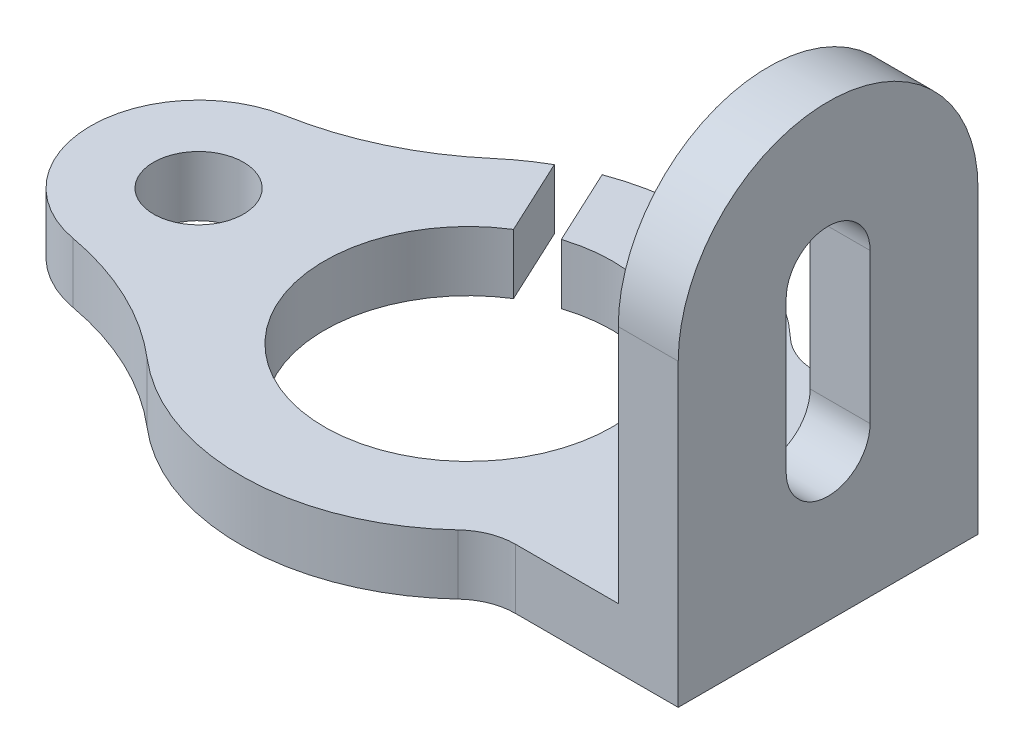
ISO-10303-21;
HEADER;
FILE_DESCRIPTION(('STEP AP214'),'2;1');
FILE_NAME('part.step','',(''),(''),'','','');
FILE_SCHEMA(('AUTOMOTIVE_DESIGN { 1 0 10303 214 1 1 1 1 }'));
ENDSEC;
DATA;
#1=APPLICATION_CONTEXT('core data for automotive mechanical design processes');
#2=APPLICATION_PROTOCOL_DEFINITION('international standard','automotive_design',2000,#1);
#3=PRODUCT_CONTEXT('',#1,'mechanical');
#4=PRODUCT('Part','Part','',(#3));
#5=PRODUCT_RELATED_PRODUCT_CATEGORY('part','',(#4));
#6=PRODUCT_DEFINITION_FORMATION('','',#4);
#7=PRODUCT_DEFINITION_CONTEXT('part definition',#1,'design');
#8=PRODUCT_DEFINITION('design','',#6,#7);
#9=PRODUCT_DEFINITION_SHAPE('','',#8);
#10=(LENGTH_UNIT() NAMED_UNIT(*) SI_UNIT(.MILLI.,.METRE.));
#11=(NAMED_UNIT(*) PLANE_ANGLE_UNIT() SI_UNIT($,.RADIAN.));
#12=(NAMED_UNIT(*) SI_UNIT($,.STERADIAN.) SOLID_ANGLE_UNIT());
#13=UNCERTAINTY_MEASURE_WITH_UNIT(LENGTH_MEASURE(1.E-05),#10,'distance_accuracy_value','');
#14=(GEOMETRIC_REPRESENTATION_CONTEXT(3) GLOBAL_UNCERTAINTY_ASSIGNED_CONTEXT((#13)) GLOBAL_UNIT_ASSIGNED_CONTEXT((#10,
#11,#12)) REPRESENTATION_CONTEXT('',''));
#15=CARTESIAN_POINT('',(0.,0.,0.));
#16=DIRECTION('',(0.,0.,1.));
#17=DIRECTION('',(1.,0.,0.));
#18=AXIS2_PLACEMENT_3D('',#15,#16,#17);
#19=CARTESIAN_POINT('',(0.,0.,43.));
#20=DIRECTION('',(0.,-1.,0.));
#21=DIRECTION('',(1.,0.,0.));
#22=AXIS2_PLACEMENT_3D('',#19,#20,#21);
#23=PLANE('',#22);
#24=CARTESIAN_POINT('',(-95.,0.,0.));
#25=DIRECTION('',(0.,-1.,0.));
#26=DIRECTION('',(1.,0.,0.));
#27=AXIS2_PLACEMENT_3D('',#24,#25,#26);
#28=CIRCLE('',#27,7.50000000000001);
#29=CARTESIAN_POINT('',(-102.5,0.,0.));
#30=VERTEX_POINT('',#29);
#31=EDGE_CURVE('E282',#30,#30,#28,.T.);
#32=ORIENTED_EDGE('',*,*,#31,.F.);
#33=EDGE_LOOP('',(#32));
#34=FACE_BOUND('',#33,.T.);
#35=DIRECTION('',(-1.,0.,0.));
#36=VECTOR('',#35,1.);
#37=CARTESIAN_POINT('',(0.,0.,-25.));
#38=LINE('',#37,#36);
#39=CARTESIAN_POINT('',(10.,0.,-25.));
#40=VERTEX_POINT('',#39);
#41=CARTESIAN_POINT('',(-17.1518645886863,0.,-25.));
#42=VERTEX_POINT('',#41);
#43=EDGE_CURVE('E281',#40,#42,#38,.T.);
#44=ORIENTED_EDGE('',*,*,#43,.F.);
#45=DIRECTION('',(0.,0.,-1.));
#46=VECTOR('',#45,1.);
#47=CARTESIAN_POINT('',(10.,0.,43.));
#48=LINE('',#47,#46);
#49=CARTESIAN_POINT('',(10.,0.,25.));
#50=VERTEX_POINT('',#49);
#51=EDGE_CURVE('E11',#50,#40,#48,.T.);
#52=ORIENTED_EDGE('',*,*,#51,.F.);
#53=DIRECTION('',(1.,0.,0.));
#54=VECTOR('',#53,1.);
#55=CARTESIAN_POINT('',(0.,0.,25.));
#56=LINE('',#55,#54);
#57=CARTESIAN_POINT('',(-17.1518645886863,0.,25.));
#58=VERTEX_POINT('',#57);
#59=EDGE_CURVE('E243',#58,#50,#56,.T.);
#60=ORIENTED_EDGE('',*,*,#59,.F.);
#61=CARTESIAN_POINT('',(-17.1518645886863,0.,35.));
#62=DIRECTION('',(0.,-1.,0.));
#63=DIRECTION('',(1.,0.,0.));
#64=AXIS2_PLACEMENT_3D('',#61,#62,#63);
#65=CIRCLE('',#64,10.);
#66=CARTESIAN_POINT('',(-23.99522613271,0.,27.7083333333333));
#67=VERTEX_POINT('',#66);
#68=EDGE_CURVE('E188',#67,#58,#65,.T.);
#69=ORIENTED_EDGE('',*,*,#68,.F.);
#70=CARTESIAN_POINT('',(-50.,0.,0.));
#71=DIRECTION('',(0.,-1.,0.));
#72=DIRECTION('',(1.,0.,0.));
#73=AXIS2_PLACEMENT_3D('',#70,#71,#72);
#74=CIRCLE('',#73,38.);
#75=CARTESIAN_POINT('',(-74.685606060606,0.,28.8898053544943));
#76=VERTEX_POINT('',#75);
#77=EDGE_CURVE('E263',#76,#67,#74,.F.);
#78=ORIENTED_EDGE('',*,*,#77,.F.);
#79=CARTESIAN_POINT('',(-107.166666666667,0.,66.9027071367237));
#80=DIRECTION('',(0.,-1.,0.));
#81=DIRECTION('',(1.,0.,0.));
#82=AXIS2_PLACEMENT_3D('',#79,#80,#81);
#83=CIRCLE('',#82,50.);
#84=CARTESIAN_POINT('',(-98.2205882352941,0.,17.7095401244269));
#85=VERTEX_POINT('',#84);
#86=EDGE_CURVE('E264',#85,#76,#83,.T.);
#87=ORIENTED_EDGE('',*,*,#86,.F.);
#88=CARTESIAN_POINT('',(-95.,0.,0.));
#89=DIRECTION('',(0.,-1.,0.));
#90=DIRECTION('',(1.,0.,0.));
#91=AXIS2_PLACEMENT_3D('',#88,#89,#90);
#92=CIRCLE('',#91,18.);
#93=CARTESIAN_POINT('',(-98.2205882352941,0.,-17.7095401244269));
#94=VERTEX_POINT('',#93);
#95=EDGE_CURVE('E270',#94,#85,#92,.F.);
#96=ORIENTED_EDGE('',*,*,#95,.F.);
#97=CARTESIAN_POINT('',(-107.166666666667,0.,-66.9027071367237));
#98=DIRECTION('',(0.,-1.,0.));
#99=DIRECTION('',(1.,0.,0.));
#100=AXIS2_PLACEMENT_3D('',#97,#98,#99);
#101=CIRCLE('',#100,50.);
#102=CARTESIAN_POINT('',(-74.685606060606,0.,-28.8898053544943));
#103=VERTEX_POINT('',#102);
#104=EDGE_CURVE('E267',#103,#94,#101,.T.);
#105=ORIENTED_EDGE('',*,*,#104,.F.);
#106=CARTESIAN_POINT('',(-50.,0.,0.));
#107=DIRECTION('',(0.,-1.,0.));
#108=DIRECTION('',(1.,0.,0.));
#109=AXIS2_PLACEMENT_3D('',#106,#107,#108);
#110=CIRCLE('',#109,38.);
#111=CARTESIAN_POINT('',(-68.7282921822066,0.,-33.0643474446102));
#112=VERTEX_POINT('',#111);
#113=EDGE_CURVE('E271',#112,#103,#110,.F.);
#114=ORIENTED_EDGE('',*,*,#113,.F.);
#115=DIRECTION('',(-0.422618261740693,0.,-0.906307787036653));
#116=VECTOR('',#115,1.);
#117=CARTESIAN_POINT('',(-27.3186580762159,0.,55.7388994714571));
#118=LINE('',#117,#116);
#119=CARTESIAN_POINT('',(-62.7822087418325,0.,-20.3129303568004));
#120=VERTEX_POINT('',#119);
#121=EDGE_CURVE('E272',#120,#112,#118,.T.);
#122=ORIENTED_EDGE('',*,*,#121,.F.);
#123=CARTESIAN_POINT('',(-50.,0.,0.));
#124=DIRECTION('',(0.,-1.,0.));
#125=DIRECTION('',(1.,0.,0.));
#126=AXIS2_PLACEMENT_3D('',#123,#124,#125);
#127=CIRCLE('',#126,24.);
#128=CARTESIAN_POINT('',(-57.3443620196126,0.,-22.8486399272445));
#129=VERTEX_POINT('',#128);
#130=EDGE_CURVE('E274',#129,#120,#127,.T.);
#131=ORIENTED_EDGE('',*,*,#130,.F.);
#132=DIRECTION('',(0.422618261740694,0.,0.906307787036653));
#133=VECTOR('',#132,1.);
#134=CARTESIAN_POINT('',(-21.8808113539959,0.,53.203189901013));
#135=LINE('',#134,#133);
#136=CARTESIAN_POINT('',(-63.2904454599867,0.,-35.6000570150543));
#137=VERTEX_POINT('',#136);
#138=EDGE_CURVE('E280',#137,#129,#135,.T.);
#139=ORIENTED_EDGE('',*,*,#138,.F.);
#140=CARTESIAN_POINT('',(-50.,0.,0.));
#141=DIRECTION('',(0.,-1.,0.));
#142=DIRECTION('',(1.,0.,0.));
#143=AXIS2_PLACEMENT_3D('',#140,#141,#142);
#144=CIRCLE('',#143,38.);
#145=CARTESIAN_POINT('',(-23.99522613271,0.,-27.7083333333333));
#146=VERTEX_POINT('',#145);
#147=EDGE_CURVE('E276',#146,#137,#144,.F.);
#148=ORIENTED_EDGE('',*,*,#147,.F.);
#149=CARTESIAN_POINT('',(-17.1518645886863,0.,-35.));
#150=DIRECTION('',(0.,-1.,0.));
#151=DIRECTION('',(1.,0.,0.));
#152=AXIS2_PLACEMENT_3D('',#149,#150,#151);
#153=CIRCLE('',#152,10.);
#154=EDGE_CURVE('E283',#42,#146,#153,.T.);
#155=ORIENTED_EDGE('',*,*,#154,.F.);
#156=EDGE_LOOP('',(#44,#52,#60,#69,#78,#87,#96,#105,#114,#122,#131,#139,#148,#155));
#157=FACE_BOUND('',#156,.T.);
#158=ADVANCED_FACE('F41',(#34,#157),#23,.T.);
#159=CARTESIAN_POINT('',(10.,0.,43.));
#160=DIRECTION('',(-1.,0.,0.));
#161=DIRECTION('',(0.,-1.,0.));
#162=AXIS2_PLACEMENT_3D('',#159,#160,#161);
#163=PLANE('',#162);
#164=ORIENTED_EDGE('',*,*,#51,.T.);
#165=DIRECTION('',(0.,1.,0.));
#166=VECTOR('',#165,1.);
#167=CARTESIAN_POINT('',(10.,0.,-25.));
#168=LINE('',#167,#166);
#169=CARTESIAN_POINT('',(10.,50.,-25.));
#170=VERTEX_POINT('',#169);
#171=EDGE_CURVE('E328',#40,#170,#168,.T.);
#172=ORIENTED_EDGE('',*,*,#171,.T.);
#173=CARTESIAN_POINT('',(9.99999999999998,50.,0.));
#174=DIRECTION('',(-1.,0.,0.));
#175=DIRECTION('',(0.,-1.,0.));
#176=AXIS2_PLACEMENT_3D('',#173,#174,#175);
#177=CIRCLE('',#176,25.);
#178=CARTESIAN_POINT('',(10.,50.,25.));
#179=VERTEX_POINT('',#178);
#180=EDGE_CURVE('E335',#170,#179,#177,.F.);
#181=ORIENTED_EDGE('',*,*,#180,.T.);
#182=DIRECTION('',(0.,-1.,0.));
#183=VECTOR('',#182,1.);
#184=CARTESIAN_POINT('',(10.,0.,25.));
#185=LINE('',#184,#183);
#186=EDGE_CURVE('E330',#179,#50,#185,.T.);
#187=ORIENTED_EDGE('',*,*,#186,.T.);
#188=EDGE_LOOP('',(#164,#172,#181,#187));
#189=FACE_BOUND('',#188,.T.);
#190=DIRECTION('',(0.,1.,0.));
#191=VECTOR('',#190,1.);
#192=CARTESIAN_POINT('',(10.,0.,7.00000000000001));
#193=LINE('',#192,#191);
#194=CARTESIAN_POINT('',(10.,25.,7.));
#195=VERTEX_POINT('',#194);
#196=CARTESIAN_POINT('',(10.,50.,7.));
#197=VERTEX_POINT('',#196);
#198=EDGE_CURVE('E321',#195,#197,#193,.T.);
#199=ORIENTED_EDGE('',*,*,#198,.T.);
#200=CARTESIAN_POINT('',(9.99999999999998,50.,0.));
#201=DIRECTION('',(-1.,0.,0.));
#202=DIRECTION('',(0.,-1.,0.));
#203=AXIS2_PLACEMENT_3D('',#200,#201,#202);
#204=CIRCLE('',#203,7.);
#205=CARTESIAN_POINT('',(10.,50.,-7.));
#206=VERTEX_POINT('',#205);
#207=EDGE_CURVE('E322',#197,#206,#204,.T.);
#208=ORIENTED_EDGE('',*,*,#207,.T.);
#209=DIRECTION('',(0.,-1.,0.));
#210=VECTOR('',#209,1.);
#211=CARTESIAN_POINT('',(10.,0.,-7.));
#212=LINE('',#211,#210);
#213=CARTESIAN_POINT('',(9.99999999999999,25.,-7.));
#214=VERTEX_POINT('',#213);
#215=EDGE_CURVE('E313',#206,#214,#212,.T.);
#216=ORIENTED_EDGE('',*,*,#215,.T.);
#217=CARTESIAN_POINT('',(9.99999999999999,25.,0.));
#218=DIRECTION('',(-1.,0.,0.));
#219=DIRECTION('',(0.,-1.,0.));
#220=AXIS2_PLACEMENT_3D('',#217,#218,#219);
#221=CIRCLE('',#220,7.);
#222=EDGE_CURVE('E318',#214,#195,#221,.T.);
#223=ORIENTED_EDGE('',*,*,#222,.T.);
#224=EDGE_LOOP('',(#199,#208,#216,#223));
#225=FACE_BOUND('',#224,.T.);
#226=ADVANCED_FACE('F396',(#189,#225),#163,.F.);
#227=CARTESIAN_POINT('',(0.,0.,43.));
#228=DIRECTION('',(-1.,0.,0.));
#229=DIRECTION('',(0.,-1.,0.));
#230=AXIS2_PLACEMENT_3D('',#227,#228,#229);
#231=PLANE('',#230);
#232=DIRECTION('',(0.,1.,0.));
#233=VECTOR('',#232,1.);
#234=CARTESIAN_POINT('',(0.,50.,-25.));
#235=LINE('',#234,#233);
#236=CARTESIAN_POINT('',(0.,10.,-25.));
#237=VERTEX_POINT('',#236);
#238=CARTESIAN_POINT('',(0.,50.,-25.));
#239=VERTEX_POINT('',#238);
#240=EDGE_CURVE('E292',#237,#239,#235,.T.);
#241=ORIENTED_EDGE('',*,*,#240,.F.);
#242=DIRECTION('',(0.,0.,-1.));
#243=VECTOR('',#242,1.);
#244=CARTESIAN_POINT('',(0.,10.,43.));
#245=LINE('',#244,#243);
#246=CARTESIAN_POINT('',(0.,10.,25.));
#247=VERTEX_POINT('',#246);
#248=EDGE_CURVE('E48',#247,#237,#245,.T.);
#249=ORIENTED_EDGE('',*,*,#248,.F.);
#250=DIRECTION('',(0.,-1.,0.));
#251=VECTOR('',#250,1.);
#252=CARTESIAN_POINT('',(0.,50.,25.));
#253=LINE('',#252,#251);
#254=CARTESIAN_POINT('',(0.,50.,25.));
#255=VERTEX_POINT('',#254);
#256=EDGE_CURVE('E197',#255,#247,#253,.T.);
#257=ORIENTED_EDGE('',*,*,#256,.F.);
#258=CARTESIAN_POINT('',(0.,50.,0.));
#259=DIRECTION('',(1.,0.,0.));
#260=DIRECTION('',(0.,-1.,0.));
#261=AXIS2_PLACEMENT_3D('',#258,#259,#260);
#262=CIRCLE('',#261,25.);
#263=EDGE_CURVE('E298',#239,#255,#262,.T.);
#264=ORIENTED_EDGE('',*,*,#263,.F.);
#265=EDGE_LOOP('',(#241,#249,#257,#264));
#266=FACE_BOUND('',#265,.T.);
#267=CARTESIAN_POINT('',(0.,50.,0.));
#268=DIRECTION('',(-1.,0.,0.));
#269=DIRECTION('',(0.,-1.,0.));
#270=AXIS2_PLACEMENT_3D('',#267,#268,#269);
#271=CIRCLE('',#270,7.);
#272=CARTESIAN_POINT('',(0.,50.,7.));
#273=VERTEX_POINT('',#272);
#274=CARTESIAN_POINT('',(0.,50.,-7.));
#275=VERTEX_POINT('',#274);
#276=EDGE_CURVE('E61',#273,#275,#271,.T.);
#277=ORIENTED_EDGE('',*,*,#276,.F.);
#278=DIRECTION('',(0.,1.,0.));
#279=VECTOR('',#278,1.);
#280=CARTESIAN_POINT('',(0.,50.,7.));
#281=LINE('',#280,#279);
#282=CARTESIAN_POINT('',(0.,25.,7.));
#283=VERTEX_POINT('',#282);
#284=EDGE_CURVE('E302',#283,#273,#281,.T.);
#285=ORIENTED_EDGE('',*,*,#284,.F.);
#286=CARTESIAN_POINT('',(0.,25.,0.));
#287=DIRECTION('',(-1.,0.,0.));
#288=DIRECTION('',(0.,-1.,0.));
#289=AXIS2_PLACEMENT_3D('',#286,#287,#288);
#290=CIRCLE('',#289,7.);
#291=CARTESIAN_POINT('',(0.,25.,-6.99999999999999));
#292=VERTEX_POINT('',#291);
#293=EDGE_CURVE('E305',#292,#283,#290,.T.);
#294=ORIENTED_EDGE('',*,*,#293,.F.);
#295=DIRECTION('',(0.,-1.,0.));
#296=VECTOR('',#295,1.);
#297=CARTESIAN_POINT('',(0.,50.,-7.));
#298=LINE('',#297,#296);
#299=EDGE_CURVE('E297',#275,#292,#298,.T.);
#300=ORIENTED_EDGE('',*,*,#299,.F.);
#301=EDGE_LOOP('',(#277,#285,#294,#300));
#302=FACE_BOUND('',#301,.T.);
#303=ADVANCED_FACE('F336',(#266,#302),#231,.T.);
#304=CARTESIAN_POINT('',(0.,10.,43.));
#305=DIRECTION('',(0.,-1.,0.));
#306=DIRECTION('',(1.,0.,0.));
#307=AXIS2_PLACEMENT_3D('',#304,#305,#306);
#308=PLANE('',#307);
#309=CARTESIAN_POINT('',(-95.,9.99999999999999,0.));
#310=DIRECTION('',(0.,1.,0.));
#311=DIRECTION('',(-1.,0.,0.));
#312=AXIS2_PLACEMENT_3D('',#309,#310,#311);
#313=CIRCLE('',#312,7.50000000000001);
#314=CARTESIAN_POINT('',(-102.5,9.99999999999999,0.));
#315=VERTEX_POINT('',#314);
#316=EDGE_CURVE('E203',#315,#315,#313,.T.);
#317=ORIENTED_EDGE('',*,*,#316,.F.);
#318=EDGE_LOOP('',(#317));
#319=FACE_BOUND('',#318,.T.);
#320=ORIENTED_EDGE('',*,*,#248,.T.);
#321=DIRECTION('',(1.,0.,0.));
#322=VECTOR('',#321,1.);
#323=CARTESIAN_POINT('',(10.,10.,-25.));
#324=LINE('',#323,#322);
#325=CARTESIAN_POINT('',(-17.1518645886863,10.,-25.));
#326=VERTEX_POINT('',#325);
#327=EDGE_CURVE('E193',#326,#237,#324,.T.);
#328=ORIENTED_EDGE('',*,*,#327,.F.);
#329=CARTESIAN_POINT('',(-17.1518645886863,10.,-35.));
#330=DIRECTION('',(0.,1.,0.));
#331=DIRECTION('',(-1.,0.,0.));
#332=AXIS2_PLACEMENT_3D('',#329,#330,#331);
#333=CIRCLE('',#332,10.);
#334=CARTESIAN_POINT('',(-23.99522613271,10.,-27.7083333333333));
#335=VERTEX_POINT('',#334);
#336=EDGE_CURVE('E232',#335,#326,#333,.T.);
#337=ORIENTED_EDGE('',*,*,#336,.F.);
#338=CARTESIAN_POINT('',(-50.,9.99999999999999,0.));
#339=DIRECTION('',(0.,-1.,0.));
#340=DIRECTION('',(-1.,0.,0.));
#341=AXIS2_PLACEMENT_3D('',#338,#339,#340);
#342=CIRCLE('',#341,38.);
#343=CARTESIAN_POINT('',(-63.2904454599867,9.99999999999999,-35.6000570150543));
#344=VERTEX_POINT('',#343);
#345=EDGE_CURVE('E235',#344,#335,#342,.T.);
#346=ORIENTED_EDGE('',*,*,#345,.F.);
#347=DIRECTION('',(-0.422618261740694,0.,-0.906307787036653));
#348=VECTOR('',#347,1.);
#349=CARTESIAN_POINT('',(-57.3443620196126,9.99999999999999,-22.8486399272445));
#350=LINE('',#349,#348);
#351=CARTESIAN_POINT('',(-57.3443620196126,9.99999999999999,-22.8486399272445));
#352=VERTEX_POINT('',#351);
#353=EDGE_CURVE('E229',#352,#344,#350,.T.);
#354=ORIENTED_EDGE('',*,*,#353,.F.);
#355=CARTESIAN_POINT('',(-50.,9.99999999999999,0.));
#356=DIRECTION('',(0.,1.,0.));
#357=DIRECTION('',(-1.,0.,0.));
#358=AXIS2_PLACEMENT_3D('',#355,#356,#357);
#359=CIRCLE('',#358,24.);
#360=CARTESIAN_POINT('',(-62.7822087418325,9.99999999999999,-20.3129303568004));
#361=VERTEX_POINT('',#360);
#362=EDGE_CURVE('E228',#361,#352,#359,.T.);
#363=ORIENTED_EDGE('',*,*,#362,.F.);
#364=DIRECTION('',(0.422618261740693,0.,0.906307787036653));
#365=VECTOR('',#364,1.);
#366=CARTESIAN_POINT('',(-62.7822087418325,9.99999999999999,-20.3129303568004));
#367=LINE('',#366,#365);
#368=CARTESIAN_POINT('',(-68.7282921822066,9.99999999999999,-33.0643474446102));
#369=VERTEX_POINT('',#368);
#370=EDGE_CURVE('E224',#369,#361,#367,.T.);
#371=ORIENTED_EDGE('',*,*,#370,.F.);
#372=CARTESIAN_POINT('',(-50.,9.99999999999999,0.));
#373=DIRECTION('',(0.,-1.,0.));
#374=DIRECTION('',(-1.,0.,0.));
#375=AXIS2_PLACEMENT_3D('',#372,#373,#374);
#376=CIRCLE('',#375,38.);
#377=CARTESIAN_POINT('',(-74.685606060606,9.99999999999999,-28.8898053544943));
#378=VERTEX_POINT('',#377);
#379=EDGE_CURVE('E219',#378,#369,#376,.T.);
#380=ORIENTED_EDGE('',*,*,#379,.F.);
#381=CARTESIAN_POINT('',(-107.166666666667,9.99999999999999,-66.9027071367237));
#382=DIRECTION('',(0.,1.,0.));
#383=DIRECTION('',(-1.,0.,0.));
#384=AXIS2_PLACEMENT_3D('',#381,#382,#383);
#385=CIRCLE('',#384,50.);
#386=CARTESIAN_POINT('',(-98.2205882352941,9.99999999999999,-17.7095401244269));
#387=VERTEX_POINT('',#386);
#388=EDGE_CURVE('E220',#387,#378,#385,.T.);
#389=ORIENTED_EDGE('',*,*,#388,.F.);
#390=CARTESIAN_POINT('',(-95.,9.99999999999999,0.));
#391=DIRECTION('',(0.,-1.,0.));
#392=DIRECTION('',(-1.,0.,0.));
#393=AXIS2_PLACEMENT_3D('',#390,#391,#392);
#394=CIRCLE('',#393,18.);
#395=CARTESIAN_POINT('',(-98.2205882352941,9.99999999999999,17.7095401244269));
#396=VERTEX_POINT('',#395);
#397=EDGE_CURVE('E212',#396,#387,#394,.T.);
#398=ORIENTED_EDGE('',*,*,#397,.F.);
#399=CARTESIAN_POINT('',(-107.166666666667,9.99999999999999,66.9027071367237));
#400=DIRECTION('',(0.,1.,0.));
#401=DIRECTION('',(-1.,0.,0.));
#402=AXIS2_PLACEMENT_3D('',#399,#400,#401);
#403=CIRCLE('',#402,50.);
#404=CARTESIAN_POINT('',(-74.685606060606,9.99999999999999,28.8898053544943));
#405=VERTEX_POINT('',#404);
#406=EDGE_CURVE('E208',#405,#396,#403,.T.);
#407=ORIENTED_EDGE('',*,*,#406,.F.);
#408=CARTESIAN_POINT('',(-50.,9.99999999999999,0.));
#409=DIRECTION('',(0.,-1.,0.));
#410=DIRECTION('',(-1.,0.,0.));
#411=AXIS2_PLACEMENT_3D('',#408,#409,#410);
#412=CIRCLE('',#411,38.);
#413=CARTESIAN_POINT('',(-23.99522613271,10.,27.7083333333333));
#414=VERTEX_POINT('',#413);
#415=EDGE_CURVE('E206',#414,#405,#412,.T.);
#416=ORIENTED_EDGE('',*,*,#415,.F.);
#417=CARTESIAN_POINT('',(-17.1518645886863,10.,35.));
#418=DIRECTION('',(0.,1.,0.));
#419=DIRECTION('',(-1.,0.,0.));
#420=AXIS2_PLACEMENT_3D('',#417,#418,#419);
#421=CIRCLE('',#420,10.);
#422=CARTESIAN_POINT('',(-17.1518645886863,10.,25.));
#423=VERTEX_POINT('',#422);
#424=EDGE_CURVE('E181',#423,#414,#421,.T.);
#425=ORIENTED_EDGE('',*,*,#424,.F.);
#426=DIRECTION('',(-1.,0.,0.));
#427=VECTOR('',#426,1.);
#428=CARTESIAN_POINT('',(10.,10.,25.));
#429=LINE('',#428,#427);
#430=EDGE_CURVE('E194',#247,#423,#429,.T.);
#431=ORIENTED_EDGE('',*,*,#430,.F.);
#432=EDGE_LOOP('',(#320,#328,#337,#346,#354,#363,#371,#380,#389,#398,#407,#416,#425,#431));
#433=FACE_BOUND('',#432,.T.);
#434=ADVANCED_FACE('F201',(#319,#433),#308,.F.);
#435=CARTESIAN_POINT('',(116.,50.,0.));
#436=DIRECTION('',(-1.,0.,0.));
#437=DIRECTION('',(0.,-1.,0.));
#438=AXIS2_PLACEMENT_3D('',#435,#436,#437);
#439=CYLINDRICAL_SURFACE('',#438,25.);
#440=DIRECTION('',(-1.,0.,0.));
#441=VECTOR('',#440,1.);
#442=CARTESIAN_POINT('',(116.,50.,-25.));
#443=LINE('',#442,#441);
#444=EDGE_CURVE('E286',#170,#239,#443,.T.);
#445=ORIENTED_EDGE('',*,*,#444,.T.);
#446=ORIENTED_EDGE('',*,*,#263,.T.);
#447=DIRECTION('',(-1.,0.,0.));
#448=VECTOR('',#447,1.);
#449=CARTESIAN_POINT('',(116.,50.,25.));
#450=LINE('',#449,#448);
#451=EDGE_CURVE('E289',#179,#255,#450,.T.);
#452=ORIENTED_EDGE('',*,*,#451,.F.);
#453=ORIENTED_EDGE('',*,*,#180,.F.);
#454=EDGE_LOOP('',(#445,#446,#452,#453));
#455=FACE_BOUND('',#454,.T.);
#456=ADVANCED_FACE('F400',(#455),#439,.T.);
#457=CARTESIAN_POINT('',(116.,50.,-25.));
#458=DIRECTION('',(0.,0.,1.));
#459=DIRECTION('',(0.,-1.,0.));
#460=AXIS2_PLACEMENT_3D('',#457,#458,#459);
#461=PLANE('',#460);
#462=ORIENTED_EDGE('',*,*,#171,.F.);
#463=ORIENTED_EDGE('',*,*,#43,.T.);
#464=DIRECTION('',(0.,1.,0.));
#465=VECTOR('',#464,1.);
#466=CARTESIAN_POINT('',(-17.1518645886863,-106.,-25.));
#467=LINE('',#466,#465);
#468=EDGE_CURVE('E239',#42,#326,#467,.T.);
#469=ORIENTED_EDGE('',*,*,#468,.T.);
#470=ORIENTED_EDGE('',*,*,#327,.T.);
#471=ORIENTED_EDGE('',*,*,#240,.T.);
#472=ORIENTED_EDGE('',*,*,#444,.F.);
#473=EDGE_LOOP('',(#462,#463,#469,#470,#471,#472));
#474=FACE_BOUND('',#473,.T.);
#475=ADVANCED_FACE('F341',(#474),#461,.F.);
#476=CARTESIAN_POINT('',(116.,50.,25.));
#477=DIRECTION('',(0.,0.,-1.));
#478=DIRECTION('',(-1.,0.,0.));
#479=AXIS2_PLACEMENT_3D('',#476,#477,#478);
#480=PLANE('',#479);
#481=ORIENTED_EDGE('',*,*,#451,.T.);
#482=ORIENTED_EDGE('',*,*,#256,.T.);
#483=ORIENTED_EDGE('',*,*,#430,.T.);
#484=DIRECTION('',(0.,1.,0.));
#485=VECTOR('',#484,1.);
#486=CARTESIAN_POINT('',(-17.1518645886863,-106.,25.));
#487=LINE('',#486,#485);
#488=EDGE_CURVE('E176',#58,#423,#487,.T.);
#489=ORIENTED_EDGE('',*,*,#488,.F.);
#490=ORIENTED_EDGE('',*,*,#59,.T.);
#491=ORIENTED_EDGE('',*,*,#186,.F.);
#492=EDGE_LOOP('',(#481,#482,#483,#489,#490,#491));
#493=FACE_BOUND('',#492,.T.);
#494=ADVANCED_FACE('F192',(#493),#480,.F.);
#495=CARTESIAN_POINT('',(116.,50.,0.));
#496=DIRECTION('',(-1.,0.,0.));
#497=DIRECTION('',(0.,-1.,0.));
#498=AXIS2_PLACEMENT_3D('',#495,#496,#497);
#499=CYLINDRICAL_SURFACE('',#498,7.);
#500=DIRECTION('',(-1.,0.,0.));
#501=VECTOR('',#500,1.);
#502=CARTESIAN_POINT('',(116.,50.,7.));
#503=LINE('',#502,#501);
#504=EDGE_CURVE('E310',#197,#273,#503,.T.);
#505=ORIENTED_EDGE('',*,*,#504,.T.);
#506=ORIENTED_EDGE('',*,*,#276,.T.);
#507=DIRECTION('',(-1.,0.,0.));
#508=VECTOR('',#507,1.);
#509=CARTESIAN_POINT('',(116.,50.,-7.));
#510=LINE('',#509,#508);
#511=EDGE_CURVE('E306',#206,#275,#510,.T.);
#512=ORIENTED_EDGE('',*,*,#511,.F.);
#513=ORIENTED_EDGE('',*,*,#207,.F.);
#514=EDGE_LOOP('',(#505,#506,#512,#513));
#515=FACE_BOUND('',#514,.T.);
#516=ADVANCED_FACE('F413',(#515),#499,.F.);
#517=CARTESIAN_POINT('',(116.,50.,7.));
#518=DIRECTION('',(0.,0.,1.));
#519=DIRECTION('',(0.,-1.,0.));
#520=AXIS2_PLACEMENT_3D('',#517,#518,#519);
#521=PLANE('',#520);
#522=DIRECTION('',(-1.,0.,0.));
#523=VECTOR('',#522,1.);
#524=CARTESIAN_POINT('',(116.,25.,7.));
#525=LINE('',#524,#523);
#526=EDGE_CURVE('E315',#195,#283,#525,.T.);
#527=ORIENTED_EDGE('',*,*,#526,.T.);
#528=ORIENTED_EDGE('',*,*,#284,.T.);
#529=ORIENTED_EDGE('',*,*,#504,.F.);
#530=ORIENTED_EDGE('',*,*,#198,.F.);
#531=EDGE_LOOP('',(#527,#528,#529,#530));
#532=FACE_BOUND('',#531,.T.);
#533=ADVANCED_FACE('F404',(#532),#521,.F.);
#534=CARTESIAN_POINT('',(116.,25.,0.));
#535=DIRECTION('',(-1.,0.,0.));
#536=DIRECTION('',(0.,-1.,0.));
#537=AXIS2_PLACEMENT_3D('',#534,#535,#536);
#538=CYLINDRICAL_SURFACE('',#537,7.);
#539=DIRECTION('',(-1.,0.,0.));
#540=VECTOR('',#539,1.);
#541=CARTESIAN_POINT('',(116.,25.,-6.99999999999999));
#542=LINE('',#541,#540);
#543=EDGE_CURVE('E54',#214,#292,#542,.T.);
#544=ORIENTED_EDGE('',*,*,#543,.T.);
#545=ORIENTED_EDGE('',*,*,#293,.T.);
#546=ORIENTED_EDGE('',*,*,#526,.F.);
#547=ORIENTED_EDGE('',*,*,#222,.F.);
#548=EDGE_LOOP('',(#544,#545,#546,#547));
#549=FACE_BOUND('',#548,.T.);
#550=ADVANCED_FACE('F408',(#549),#538,.F.);
#551=CARTESIAN_POINT('',(116.,50.,-7.));
#552=DIRECTION('',(0.,0.,-1.));
#553=DIRECTION('',(0.,1.,0.));
#554=AXIS2_PLACEMENT_3D('',#551,#552,#553);
#555=PLANE('',#554);
#556=ORIENTED_EDGE('',*,*,#511,.T.);
#557=ORIENTED_EDGE('',*,*,#299,.T.);
#558=ORIENTED_EDGE('',*,*,#543,.F.);
#559=ORIENTED_EDGE('',*,*,#215,.F.);
#560=EDGE_LOOP('',(#556,#557,#558,#559));
#561=FACE_BOUND('',#560,.T.);
#562=ADVANCED_FACE('F407',(#561),#555,.F.);
#563=CARTESIAN_POINT('',(-17.1518645886863,-106.,-35.));
#564=DIRECTION('',(0.,1.,0.));
#565=DIRECTION('',(-1.,0.,0.));
#566=AXIS2_PLACEMENT_3D('',#563,#564,#565);
#567=CYLINDRICAL_SURFACE('',#566,10.);
#568=ORIENTED_EDGE('',*,*,#154,.T.);
#569=DIRECTION('',(0.,1.,0.));
#570=VECTOR('',#569,1.);
#571=CARTESIAN_POINT('',(-23.99522613271,-106.,-27.7083333333333));
#572=LINE('',#571,#570);
#573=EDGE_CURVE('E245',#146,#335,#572,.T.);
#574=ORIENTED_EDGE('',*,*,#573,.T.);
#575=ORIENTED_EDGE('',*,*,#336,.T.);
#576=ORIENTED_EDGE('',*,*,#468,.F.);
#577=EDGE_LOOP('',(#568,#574,#575,#576));
#578=FACE_BOUND('',#577,.T.);
#579=ADVANCED_FACE('F346',(#578),#567,.F.);
#580=CARTESIAN_POINT('',(-50.,-106.,0.));
#581=DIRECTION('',(0.,1.,0.));
#582=DIRECTION('',(-1.,0.,0.));
#583=AXIS2_PLACEMENT_3D('',#580,#581,#582);
#584=CYLINDRICAL_SURFACE('',#583,38.);
#585=ORIENTED_EDGE('',*,*,#147,.T.);
#586=DIRECTION('',(0.,1.,0.));
#587=VECTOR('',#586,1.);
#588=CARTESIAN_POINT('',(-63.2904454599866,-106.,-35.6000570150543));
#589=LINE('',#588,#587);
#590=EDGE_CURVE('E244',#137,#344,#589,.T.);
#591=ORIENTED_EDGE('',*,*,#590,.T.);
#592=ORIENTED_EDGE('',*,*,#345,.T.);
#593=ORIENTED_EDGE('',*,*,#573,.F.);
#594=EDGE_LOOP('',(#585,#591,#592,#593));
#595=FACE_BOUND('',#594,.T.);
#596=ADVANCED_FACE('F354',(#595),#584,.T.);
#597=CARTESIAN_POINT('',(-57.3443620196125,-106.,-22.8486399272445));
#598=DIRECTION('',(0.906307787036653,0.,-0.422618261740694));
#599=DIRECTION('',(-0.422618261740694,0.,-0.906307787036653));
#600=AXIS2_PLACEMENT_3D('',#597,#598,#599);
#601=PLANE('',#600);
#602=ORIENTED_EDGE('',*,*,#138,.T.);
#603=DIRECTION('',(0.,1.,0.));
#604=VECTOR('',#603,1.);
#605=CARTESIAN_POINT('',(-57.3443620196125,-106.,-22.8486399272445));
#606=LINE('',#605,#604);
#607=EDGE_CURVE('E248',#129,#352,#606,.T.);
#608=ORIENTED_EDGE('',*,*,#607,.T.);
#609=ORIENTED_EDGE('',*,*,#353,.T.);
#610=ORIENTED_EDGE('',*,*,#590,.F.);
#611=EDGE_LOOP('',(#602,#608,#609,#610));
#612=FACE_BOUND('',#611,.T.);
#613=ADVANCED_FACE('F359',(#612),#601,.F.);
#614=CARTESIAN_POINT('',(-50.,-106.,0.));
#615=DIRECTION('',(0.,1.,0.));
#616=DIRECTION('',(-1.,0.,0.));
#617=AXIS2_PLACEMENT_3D('',#614,#615,#616);
#618=CYLINDRICAL_SURFACE('',#617,24.);
#619=ORIENTED_EDGE('',*,*,#130,.T.);
#620=DIRECTION('',(0.,1.,0.));
#621=VECTOR('',#620,1.);
#622=CARTESIAN_POINT('',(-62.7822087418324,-106.,-20.3129303568004));
#623=LINE('',#622,#621);
#624=EDGE_CURVE('E246',#120,#361,#623,.T.);
#625=ORIENTED_EDGE('',*,*,#624,.T.);
#626=ORIENTED_EDGE('',*,*,#362,.T.);
#627=ORIENTED_EDGE('',*,*,#607,.F.);
#628=EDGE_LOOP('',(#619,#625,#626,#627));
#629=FACE_BOUND('',#628,.T.);
#630=ADVANCED_FACE('F361',(#629),#618,.F.);
#631=CARTESIAN_POINT('',(-62.7822087418324,-106.,-20.3129303568004));
#632=DIRECTION('',(-0.906307787036653,0.,0.422618261740693));
#633=DIRECTION('',(0.422618261740693,0.,0.906307787036653));
#634=AXIS2_PLACEMENT_3D('',#631,#632,#633);
#635=PLANE('',#634);
#636=ORIENTED_EDGE('',*,*,#121,.T.);
#637=DIRECTION('',(0.,1.,0.));
#638=VECTOR('',#637,1.);
#639=CARTESIAN_POINT('',(-68.7282921822066,-106.,-33.0643474446102));
#640=LINE('',#639,#638);
#641=EDGE_CURVE('E247',#112,#369,#640,.T.);
#642=ORIENTED_EDGE('',*,*,#641,.T.);
#643=ORIENTED_EDGE('',*,*,#370,.T.);
#644=ORIENTED_EDGE('',*,*,#624,.F.);
#645=EDGE_LOOP('',(#636,#642,#643,#644));
#646=FACE_BOUND('',#645,.T.);
#647=ADVANCED_FACE('F369',(#646),#635,.F.);
#648=CARTESIAN_POINT('',(-50.,-106.,0.));
#649=DIRECTION('',(0.,1.,0.));
#650=DIRECTION('',(-1.,0.,0.));
#651=AXIS2_PLACEMENT_3D('',#648,#649,#650);
#652=CYLINDRICAL_SURFACE('',#651,38.);
#653=ORIENTED_EDGE('',*,*,#113,.T.);
#654=DIRECTION('',(0.,1.,0.));
#655=VECTOR('',#654,1.);
#656=CARTESIAN_POINT('',(-74.685606060606,-106.,-28.8898053544943));
#657=LINE('',#656,#655);
#658=EDGE_CURVE('E252',#103,#378,#657,.T.);
#659=ORIENTED_EDGE('',*,*,#658,.T.);
#660=ORIENTED_EDGE('',*,*,#379,.T.);
#661=ORIENTED_EDGE('',*,*,#641,.F.);
#662=EDGE_LOOP('',(#653,#659,#660,#661));
#663=FACE_BOUND('',#662,.T.);
#664=ADVANCED_FACE('F372',(#663),#652,.T.);
#665=CARTESIAN_POINT('',(-107.166666666667,-106.,-66.9027071367237));
#666=DIRECTION('',(0.,1.,0.));
#667=DIRECTION('',(-1.,0.,0.));
#668=AXIS2_PLACEMENT_3D('',#665,#666,#667);
#669=CYLINDRICAL_SURFACE('',#668,50.);
#670=ORIENTED_EDGE('',*,*,#104,.T.);
#671=DIRECTION('',(0.,1.,0.));
#672=VECTOR('',#671,1.);
#673=CARTESIAN_POINT('',(-98.2205882352941,-106.,-17.7095401244269));
#674=LINE('',#673,#672);
#675=EDGE_CURVE('E255',#94,#387,#674,.T.);
#676=ORIENTED_EDGE('',*,*,#675,.T.);
#677=ORIENTED_EDGE('',*,*,#388,.T.);
#678=ORIENTED_EDGE('',*,*,#658,.F.);
#679=EDGE_LOOP('',(#670,#676,#677,#678));
#680=FACE_BOUND('',#679,.T.);
#681=ADVANCED_FACE('F378',(#680),#669,.F.);
#682=CARTESIAN_POINT('',(-95.,-106.,0.));
#683=DIRECTION('',(0.,1.,0.));
#684=DIRECTION('',(-1.,0.,0.));
#685=AXIS2_PLACEMENT_3D('',#682,#683,#684);
#686=CYLINDRICAL_SURFACE('',#685,18.);
#687=ORIENTED_EDGE('',*,*,#95,.T.);
#688=DIRECTION('',(0.,1.,0.));
#689=VECTOR('',#688,1.);
#690=CARTESIAN_POINT('',(-98.2205882352941,-106.,17.7095401244269));
#691=LINE('',#690,#689);
#692=EDGE_CURVE('E258',#85,#396,#691,.T.);
#693=ORIENTED_EDGE('',*,*,#692,.T.);
#694=ORIENTED_EDGE('',*,*,#397,.T.);
#695=ORIENTED_EDGE('',*,*,#675,.F.);
#696=EDGE_LOOP('',(#687,#693,#694,#695));
#697=FACE_BOUND('',#696,.T.);
#698=ADVANCED_FACE('F385',(#697),#686,.T.);
#699=CARTESIAN_POINT('',(-107.166666666667,-106.,66.9027071367237));
#700=DIRECTION('',(0.,1.,0.));
#701=DIRECTION('',(-1.,0.,0.));
#702=AXIS2_PLACEMENT_3D('',#699,#700,#701);
#703=CYLINDRICAL_SURFACE('',#702,50.);
#704=ORIENTED_EDGE('',*,*,#86,.T.);
#705=DIRECTION('',(0.,1.,0.));
#706=VECTOR('',#705,1.);
#707=CARTESIAN_POINT('',(-74.685606060606,-106.,28.8898053544943));
#708=LINE('',#707,#706);
#709=EDGE_CURVE('E256',#76,#405,#708,.T.);
#710=ORIENTED_EDGE('',*,*,#709,.T.);
#711=ORIENTED_EDGE('',*,*,#406,.T.);
#712=ORIENTED_EDGE('',*,*,#692,.F.);
#713=EDGE_LOOP('',(#704,#710,#711,#712));
#714=FACE_BOUND('',#713,.T.);
#715=ADVANCED_FACE('F390',(#714),#703,.F.);
#716=CARTESIAN_POINT('',(-50.,-106.,0.));
#717=DIRECTION('',(0.,1.,0.));
#718=DIRECTION('',(-1.,0.,0.));
#719=AXIS2_PLACEMENT_3D('',#716,#717,#718);
#720=CYLINDRICAL_SURFACE('',#719,38.);
#721=ORIENTED_EDGE('',*,*,#77,.T.);
#722=DIRECTION('',(0.,1.,0.));
#723=VECTOR('',#722,1.);
#724=CARTESIAN_POINT('',(-23.99522613271,-106.,27.7083333333333));
#725=LINE('',#724,#723);
#726=EDGE_CURVE('E187',#67,#414,#725,.T.);
#727=ORIENTED_EDGE('',*,*,#726,.T.);
#728=ORIENTED_EDGE('',*,*,#415,.T.);
#729=ORIENTED_EDGE('',*,*,#709,.F.);
#730=EDGE_LOOP('',(#721,#727,#728,#729));
#731=FACE_BOUND('',#730,.T.);
#732=ADVANCED_FACE('F393',(#731),#720,.T.);
#733=CARTESIAN_POINT('',(-17.1518645886863,-106.,35.));
#734=DIRECTION('',(0.,1.,0.));
#735=DIRECTION('',(-1.,0.,0.));
#736=AXIS2_PLACEMENT_3D('',#733,#734,#735);
#737=CYLINDRICAL_SURFACE('',#736,10.);
#738=ORIENTED_EDGE('',*,*,#68,.T.);
#739=ORIENTED_EDGE('',*,*,#488,.T.);
#740=ORIENTED_EDGE('',*,*,#424,.T.);
#741=ORIENTED_EDGE('',*,*,#726,.F.);
#742=EDGE_LOOP('',(#738,#739,#740,#741));
#743=FACE_BOUND('',#742,.T.);
#744=ADVANCED_FACE('F177',(#743),#737,.F.);
#745=CARTESIAN_POINT('',(-95.,-106.,0.));
#746=DIRECTION('',(0.,1.,0.));
#747=DIRECTION('',(-1.,0.,0.));
#748=AXIS2_PLACEMENT_3D('',#745,#746,#747);
#749=CYLINDRICAL_SURFACE('',#748,7.50000000000001);
#750=CARTESIAN_POINT('',(-102.5,0.,0.));
#751=CARTESIAN_POINT('',(-102.5,0.104166666666651,0.));
#752=CARTESIAN_POINT('',(-102.5,0.208333333333315,0.));
#753=CARTESIAN_POINT('',(-102.5,0.416666666666649,0.));
#754=CARTESIAN_POINT('',(-102.5,0.520833333333318,0.));
#755=CARTESIAN_POINT('',(-102.5,0.729166666666656,0.));
#756=CARTESIAN_POINT('',(-102.5,0.833333333333325,0.));
#757=CARTESIAN_POINT('',(-102.5,1.04166666666666,0.));
#758=CARTESIAN_POINT('',(-102.5,1.14583333333332,0.));
#759=CARTESIAN_POINT('',(-102.5,1.35416666666665,0.));
#760=CARTESIAN_POINT('',(-102.5,1.45833333333332,0.));
#761=CARTESIAN_POINT('',(-102.5,1.66666666666665,0.));
#762=CARTESIAN_POINT('',(-102.5,1.77083333333332,0.));
#763=CARTESIAN_POINT('',(-102.5,1.97916666666666,0.));
#764=CARTESIAN_POINT('',(-102.5,2.08333333333333,0.));
#765=CARTESIAN_POINT('',(-102.5,2.29166666666666,0.));
#766=CARTESIAN_POINT('',(-102.5,2.39583333333332,0.));
#767=CARTESIAN_POINT('',(-102.5,2.60416666666665,0.));
#768=CARTESIAN_POINT('',(-102.5,2.70833333333332,0.));
#769=CARTESIAN_POINT('',(-102.5,2.91666666666665,0.));
#770=CARTESIAN_POINT('',(-102.5,3.02083333333332,0.));
#771=CARTESIAN_POINT('',(-102.5,3.22916666666666,0.));
#772=CARTESIAN_POINT('',(-102.5,3.33333333333333,0.));
#773=CARTESIAN_POINT('',(-102.5,3.54166666666666,0.));
#774=CARTESIAN_POINT('',(-102.5,3.64583333333333,0.));
#775=CARTESIAN_POINT('',(-102.5,3.85416666666665,0.));
#776=CARTESIAN_POINT('',(-102.5,3.95833333333332,0.));
#777=CARTESIAN_POINT('',(-102.5,4.16666666666665,0.));
#778=CARTESIAN_POINT('',(-102.5,4.27083333333332,0.));
#779=CARTESIAN_POINT('',(-102.5,4.47916666666666,0.));
#780=CARTESIAN_POINT('',(-102.5,4.58333333333333,0.));
#781=CARTESIAN_POINT('',(-102.5,4.79166666666666,0.));
#782=CARTESIAN_POINT('',(-102.5,4.89583333333333,0.));
#783=CARTESIAN_POINT('',(-102.5,5.10416666666666,0.));
#784=CARTESIAN_POINT('',(-102.5,5.20833333333332,0.));
#785=CARTESIAN_POINT('',(-102.5,5.41666666666665,0.));
#786=CARTESIAN_POINT('',(-102.5,5.52083333333332,0.));
#787=CARTESIAN_POINT('',(-102.5,5.72916666666666,0.));
#788=CARTESIAN_POINT('',(-102.5,5.83333333333333,0.));
#789=CARTESIAN_POINT('',(-102.5,6.04166666666666,0.));
#790=CARTESIAN_POINT('',(-102.5,6.14583333333333,0.));
#791=CARTESIAN_POINT('',(-102.5,6.35416666666666,0.));
#792=CARTESIAN_POINT('',(-102.5,6.45833333333332,0.));
#793=CARTESIAN_POINT('',(-102.5,6.66666666666665,0.));
#794=CARTESIAN_POINT('',(-102.5,6.77083333333332,0.));
#795=CARTESIAN_POINT('',(-102.5,6.97916666666666,0.));
#796=CARTESIAN_POINT('',(-102.5,7.08333333333333,0.));
#797=CARTESIAN_POINT('',(-102.5,7.29166666666666,0.));
#798=CARTESIAN_POINT('',(-102.5,7.39583333333333,0.));
#799=CARTESIAN_POINT('',(-102.5,7.60416666666666,0.));
#800=CARTESIAN_POINT('',(-102.5,7.70833333333332,0.));
#801=CARTESIAN_POINT('',(-102.5,7.91666666666666,0.));
#802=CARTESIAN_POINT('',(-102.5,8.02083333333333,0.));
#803=CARTESIAN_POINT('',(-102.5,8.22916666666666,0.));
#804=CARTESIAN_POINT('',(-102.5,8.33333333333333,0.));
#805=CARTESIAN_POINT('',(-102.5,8.54166666666666,0.));
#806=CARTESIAN_POINT('',(-102.5,8.64583333333333,0.));
#807=CARTESIAN_POINT('',(-102.5,8.85416666666666,0.));
#808=CARTESIAN_POINT('',(-102.5,8.95833333333332,0.));
#809=CARTESIAN_POINT('',(-102.5,9.16666666666666,0.));
#810=CARTESIAN_POINT('',(-102.5,9.27083333333333,0.));
#811=CARTESIAN_POINT('',(-102.5,9.47916666666666,0.));
#812=CARTESIAN_POINT('',(-102.5,9.58333333333333,0.));
#813=CARTESIAN_POINT('',(-102.5,9.79166666666667,0.));
#814=CARTESIAN_POINT('',(-102.5,9.89583333333333,0.));
#815=CARTESIAN_POINT('',(-102.5,9.99999999999999,0.));
#816=B_SPLINE_CURVE_WITH_KNOTS('',3,(#750,#751,#752,#753,#754,#755,#756,#757,#758,#759,#760,
#761,#762,#763,#764,#765,#766,#767,#768,#769,#770,#771,#772,#773,#774,#775,#776,#777,#778,#779,
#780,#781,#782,#783,#784,#785,#786,#787,#788,#789,#790,#791,#792,#793,#794,#795,#796,#797,#798,
#799,#800,#801,#802,#803,#804,#805,#806,#807,#808,#809,#810,#811,#812,#813,#814,#815),
.UNSPECIFIED.,.F.,.F.,(4,2,2,2,2,2,2,2,2,2,2,2,2,2,2,2,2,2,2,2,2,2,2,2,2,2,2,2,2,2,2,2,4),(0.,
0.312499999999993,0.625000000000001,0.937500000000008,1.25,1.56249999999999,1.875,
2.18750000000001,2.5,2.8125,3.125,3.43750000000001,3.75,4.0625,4.375,4.68750000000001,5.,5.3125,
5.62500000000001,5.93750000000001,6.25000000000001,6.5625,6.87500000000001,7.18750000000001,
7.50000000000001,7.8125,8.12500000000001,8.43750000000001,8.75000000000001,9.0625,
9.37500000000001,9.68750000000002,10.),.UNSPECIFIED.);
#817=EDGE_CURVE('BSEAM429',#30,#315,#816,.T.);
#818=ORIENTED_EDGE('',*,*,#31,.T.);
#819=ORIENTED_EDGE('',*,*,#316,.T.);
#820=ORIENTED_EDGE('',*,*,#817,.T.);
#821=ORIENTED_EDGE('',*,*,#817,.F.);
#822=EDGE_LOOP('',(#818,#820,#819,#821));
#823=FACE_BOUND('',#822,.T.);
#824=ADVANCED_FACE('F429',(#823),#749,.F.);
#825=CLOSED_SHELL('',(#158,#226,#303,#434,#456,#475,#494,#516,#533,#550,#562,#579,#596,#613,
#630,#647,#664,#681,#698,#715,#732,#744,#824));
#826=MANIFOLD_SOLID_BREP('B2',#825);
#827=ADVANCED_BREP_SHAPE_REPRESENTATION('',(#18,#826),#14);
#828=SHAPE_DEFINITION_REPRESENTATION(#9,#827);
ENDSEC;
END-ISO-10303-21;
